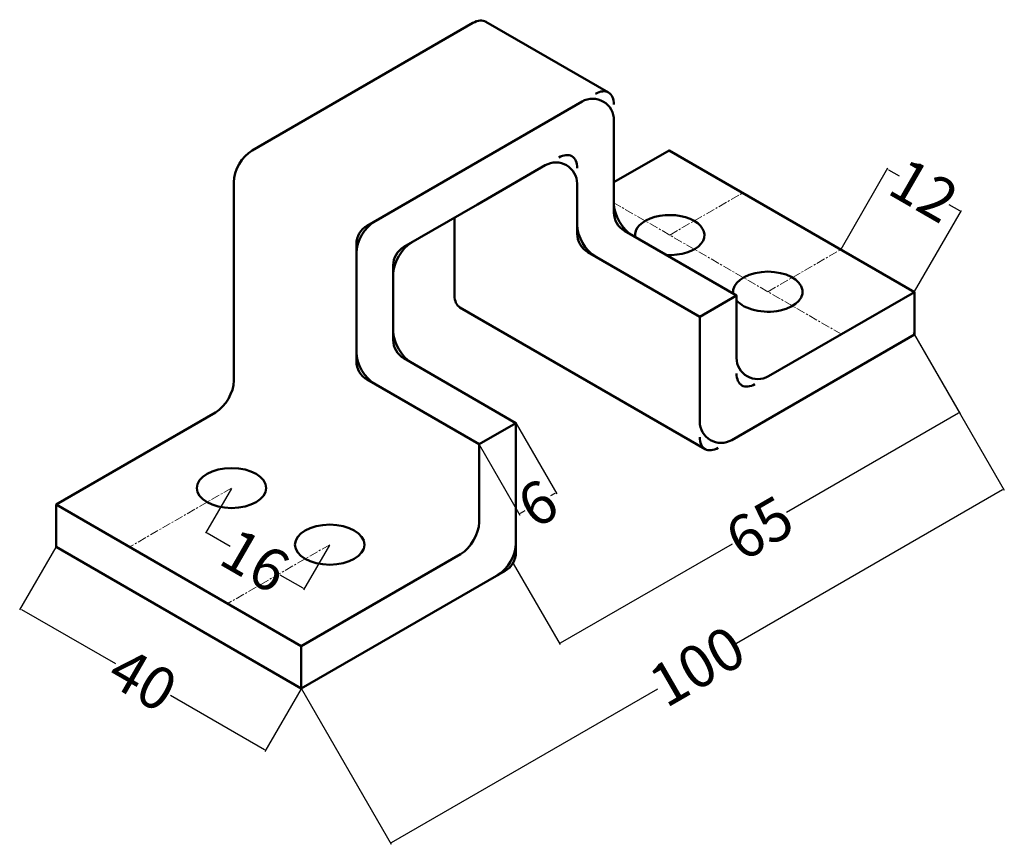
# Model space of a CAD drawing. Units: millimetres. Extents: x -15 to 124, y 15 to 131.
import ezdxf

# ---------------------------------------------------------------- set-up
doc = ezdxf.new("R2010")
doc.units = ezdxf.units.MM
doc.header["$MEASUREMENT"] = 0
doc.linetypes.add('CENTER', pattern=[2, 1.25, -0.25, 0.25, -0.25])
for name, color, linetype, lineweight in [('M-CNTR', 1, 'CENTER', 18), ('M-DIMS', 2, 'Continuous', 25), ('M-OUTL', 7, 'Continuous', 50)]:
    doc.layers.add(name, color=color, linetype=linetype, lineweight=lineweight)
doc.styles.get("Standard").update_dxf_attribs({"font": 'arial.ttf'})
doc.dimstyles.get("Standard").update_dxf_attribs({"dimtxt": 6, "dimasz": 0.18, "dimexe": 0.18, "dimexo": 0.0625, "dimgap": 0.09, "dimtad": 0, "dimtoh": 1, "dimdec": 0, "dimzin": 0, "dimdsep": 46, "dimtxsty": 'Standard', "dimcen": 0.09, "dimadec": 0, "dimazin": 0, "dimtfac": 1, "dimtdec": 0, "dimtofl": 0, "dimtmove": 0, "dimatfit": 3, "dimfxl": 1, "dimtolj": 1, "dimtzin": 0, "dimarcsym": 0})

# ---------------------------------------------------------------- blocks, each defined once
blk = doc.blocks.new('*D1')
at = {"layer": 'Defpoints', "color": 0, "transparency": 16777216}
for p in [(111.54, 86.71), (124.15, 64.87), (24.94, 36.71)]:
    blk.add_point(p, dxfattribs=at)
at = {"layer": 'M-DIMS', "color": 0, "lineweight": -2, "transparency": 16777216}
for p, q in [((111.57, 86.66), (124.24, 64.71)), ((123.99, 64.78), (86.41, 43.08)), ((24.97, 36.66), (37.64, 14.71)), ((37.7, 14.96), (75.28, 36.66))]:
    blk.add_line(p, q, dxfattribs=at)
at = {"layer": 'M-DIMS', "color": 0, "transparency": 16777216}
for points in [[(123.98, 64.81), (124.01, 64.75), (124.15, 64.87)], [(37.69, 14.99), (37.72, 14.93), (37.55, 14.87)]]:
    blk.add_solid(points, dxfattribs=at)
at = {"layer": 'M-DIMS', "color": 0, "transparency": 16777216, "insert": (80.85, 39.87), "char_height": 6, "attachment_point": 5, "rotation": 30}
blk.add_mtext('\\A1;100', dxfattribs=at)
blk = doc.blocks.new('*D2')
at = {"layer": 'Defpoints', "color": 0, "transparency": 16777216}
for p in [(111.34, 87.06), (117.91, 75.69), (54.85, 54.44)]:
    blk.add_point(p, dxfattribs=at)
at = {"layer": 'M-DIMS', "color": 0, "lineweight": -2, "transparency": 16777216}
for p, q in [((111.37, 87.01), (118, 75.53)), ((117.75, 75.6), (93.49, 61.59)), ((61.57, 43.16), (85.83, 57.16)), ((54.88, 54.39), (61.5, 42.91))]:
    blk.add_line(p, q, dxfattribs=at)
at = {"layer": 'M-DIMS', "color": 0, "transparency": 16777216}
for points in [[(117.73, 75.62), (117.76, 75.57), (117.91, 75.69)], [(61.55, 43.19), (61.58, 43.13), (61.41, 43.07)]]:
    blk.add_solid(points, dxfattribs=at)
at = {"layer": 'M-DIMS', "color": 0, "transparency": 16777216, "insert": (89.66, 59.38), "char_height": 6, "attachment_point": 5, "rotation": 30}
blk.add_mtext('\\A1;65', dxfattribs=at)
blk = doc.blocks.new('*D3')
at = {"layer": 'Defpoints', "color": 0, "transparency": 16777216}
for p in [(118.1, 104.07), (101.15, 98.71), (111.54, 92.71)]:
    blk.add_point(p, dxfattribs=at)
at = {"layer": 'M-DIMS', "color": 0, "lineweight": -2, "transparency": 16777216}
for p, q in [((101.18, 98.77), (107.79, 110.23)), ((107.86, 109.98), (109.37, 109.11)), ((117.94, 104.16), (116.43, 105.03)), ((111.57, 92.77), (118.19, 104.23))]:
    blk.add_line(p, q, dxfattribs=at)
at = {"layer": 'M-DIMS', "color": 0, "transparency": 16777216}
for points in [[(107.88, 110.01), (107.85, 109.95), (107.7, 110.07)], [(117.96, 104.19), (117.93, 104.13), (118.1, 104.07)]]:
    blk.add_solid(points, dxfattribs=at)
at = {"layer": 'M-DIMS', "color": 0, "transparency": 16777216, "insert": (112.9, 107.07), "char_height": 6, "attachment_point": 5, "rotation": 330}
blk.add_mtext('\\A1;12', dxfattribs=at)
blk = doc.blocks.new('*D4')
at = {"layer": 'Defpoints', "color": 0, "transparency": 16777216}
for p in [(15.09, 65.03), (28.95, 57.03), (25.35, 50.79)]:
    blk.add_point(p, dxfattribs=at)
at = {"layer": 'M-DIMS', "color": 0, "lineweight": -2, "transparency": 16777216}
for p, q in [((15.06, 64.97), (11.4, 58.64)), ((11.65, 58.7), (14.87, 56.84)), ((28.92, 56.97), (25.26, 50.64)), ((25.19, 50.88), (21.97, 52.74))]:
    blk.add_line(p, q, dxfattribs=at)
at = {"layer": 'M-DIMS', "color": 0, "transparency": 16777216}
for points in [[(11.66, 58.73), (11.63, 58.67), (11.49, 58.79)], [(25.21, 50.91), (25.18, 50.85), (25.35, 50.79)]]:
    blk.add_solid(points, dxfattribs=at)
at = {"layer": 'M-DIMS', "color": 0, "transparency": 16777216, "insert": (18.42, 54.79), "char_height": 6, "attachment_point": 5, "rotation": 330}
blk.add_mtext('\\A1;16', dxfattribs=at)
blk = doc.blocks.new('*D5')
at = {"layer": 'Defpoints', "color": 0, "transparency": 16777216}
for p in [(55.25, 74.21), (50.05, 71.21), (60.93, 64.37)]:
    blk.add_point(p, dxfattribs=at)
at = {"layer": 'M-DIMS', "color": 0, "lineweight": -2, "transparency": 16777216}
for p, q in [((55.28, 74.16), (61.02, 64.22)), ((50.08, 71.16), (55.82, 61.22)), ((60.77, 64.28), (60.12, 63.91)), ((55.89, 61.46), (56.54, 61.84))]:
    blk.add_line(p, q, dxfattribs=at)
at = {"layer": 'M-DIMS', "color": 0, "transparency": 16777216}
for points in [[(60.76, 64.31), (60.79, 64.26), (60.93, 64.37)], [(55.87, 61.49), (55.9, 61.44), (55.73, 61.37)]]:
    blk.add_solid(points, dxfattribs=at)
at = {"layer": 'M-DIMS', "color": 0, "transparency": 16777216, "insert": (58.33, 62.87), "char_height": 6, "attachment_point": 5, "rotation": 30}
blk.add_mtext('\\A1;6', dxfattribs=at)
blk = doc.blocks.new('*D6')
at = {"layer": 'Defpoints', "color": 0, "transparency": 16777216}
for p in [(-9.7, 56.71), (24.94, 36.71), (19.9, 27.98)]:
    blk.add_point(p, dxfattribs=at)
at = {"layer": 'M-DIMS', "color": 0, "lineweight": -2, "transparency": 16777216}
for p, q in [((-9.74, 56.66), (-14.84, 47.82)), ((-14.59, 47.89), (-1.32, 40.23)), ((24.91, 36.66), (19.81, 27.82)), ((19.74, 28.07), (6.47, 35.73))]:
    blk.add_line(p, q, dxfattribs=at)
at = {"layer": 'M-DIMS', "color": 0, "transparency": 16777216}
for points in [[(-14.57, 47.92), (-14.6, 47.86), (-14.75, 47.98)], [(19.75, 28.1), (19.72, 28.04), (19.9, 27.98)]]:
    blk.add_solid(points, dxfattribs=at)
at = {"layer": 'M-DIMS', "color": 0, "transparency": 16777216, "insert": (2.57, 37.98), "char_height": 6, "attachment_point": 5, "rotation": 330}
blk.add_mtext('\\A1;40', dxfattribs=at)

msp = doc.modelspace()

# ---------------------------------------------------------------- linework, layer by layer
at = {"layer": 'M-CNTR'}
for p, q in [((76.98, 100.76), (87.29, 106.71)), ((101.23, 86.76), (69.1, 105.31)), ((90.84, 92.76), (101.23, 98.76)), ((15.09, 65.03), (0.69, 56.71)), ((28.95, 57.03), (14.54, 48.71))]:
    msp.add_line(p, q, dxfattribs=at)
at = {"layer": 'M-OUTL'}
for p, q in [((68.34, 120.89), (51.02, 130.89)), ((18.01, 112.71), (49.19, 130.71)), ((15.41, 80.21), (15.41, 108.21)), ((46.59, 92.21), (46.59, 103.21)), ((81.99, 70.53), (47.35, 90.53)), ((-9.7, 62.71), (12.81, 75.71)), ((50.05, 60.21), (50.05, 71.21)), ((24.94, 42.71), (-9.7, 62.71)), ((24.94, 42.71), (47.45, 55.71))]:
    msp.add_line(p, q, dxfattribs=at)
for points in [[(69.1, 108.21), (76.9, 112.71), (111.54, 92.71), (90.92, 80.81, -0.57735), (86.42, 83.41), (86.42, 92.21), (81.23, 89.21), (65.41, 98.35, -0.267949), (63.91, 100.94), (63.91, 108.02, 0.57735), (59.41, 110.61), (49.82, 105.08), (39.43, 99.08, 0.267949), (37.93, 96.48), (37.93, 85.94, 0.267949), (39.43, 83.35), (55.25, 74.21), (50.05, 71.21), (34.23, 80.35, -0.267949), (32.73, 82.94), (32.73, 99.48, -0.267949), (34.23, 102.08), (64.6, 119.61), (64.6, 119.61, -0.583481), (69.1, 116.96), (69.1, 117.02), (69.1, 103.94, 0.267949), (70.6, 101.35), (86.42, 92.21)], [(111.54, 92.71), (111.54, 86.71), (85.73, 71.81), (85.73, 71.81, -0.57735), (81.23, 74.41), (81.23, 74.41), (81.23, 89.21)], [(24.94, 36.71), (53.75, 53.35, 0.267949), (55.25, 55.94), (55.25, 74.21)]]:
    msp.add_lwpolyline(points, format="xyb", dxfattribs=at)
msp.add_lwpolyline([(-9.7, 62.71), (-9.7, 56.71), (24.94, 36.71), (24.94, 42.71)], dxfattribs=at)
for centre, major_axis, start_param, end_param in [((49.19, 127.71), (1.84, 3.18), 0, 0.785398), ((66.51, 117.71), (1.84, 3.18), 0, 0.785398), ((66.51, 117.71), (1.84, 3.18), 5.497787, 6.283185), ((18.01, 109.71), (-1.84, -3.18), 3.926991, 5.497787), ((61.31, 108.71), (1.84, 3.18), 0, 0.785398), ((61.31, 108.71), (1.84, 3.18), 5.497787, 6.283185), ((71.7, 103.71), (-1.84, 3.18), 0.785398, 2.356194), ((76.98, 100.76), (-4.9, 0), 1.47024, 6.383742), ((35.33, 99.71), (-1.84, -3.18), 3.926991, 5.497787), ((66.51, 100.71), (-1.84, 3.18), 0.785398, 2.356194), ((40.53, 96.71), (1.84, 3.18), 0.785398, 2.356194), ((90.84, 92.76), (-4.9, 0), 0.448217, 6.383742), ((49.19, 93.71), (-1.84, -3.18), 5.497787, 6.283185), ((40.53, 85.71), (-1.84, 3.18), 0.785398, 2.356194), ((35.33, 82.71), (-1.84, 3.18), 0.785398, 2.356194), ((89.02, 82.71), (1.84, 3.18), 2.356194, 3.141593), ((12.81, 78.71), (1.84, 3.18), 3.926991, 5.497787), ((89.02, 82.71), (1.84, 3.18), 3.141593, 3.926991), ((83.83, 73.71), (-1.84, -3.18), 5.497787, 6.283185), ((83.83, 73.71), (-1.84, -3.18), 0, 0.785398), ((47.45, 58.71), (1.84, 3.18), 3.926991, 5.497787), ((52.65, 55.71), (1.84, 3.18), 3.926991, 5.497787)]:
    msp.add_ellipse(centre, major_axis=major_axis, ratio=0.57735, start_param=start_param, end_param=end_param, dxfattribs=at)
for centre in [(15.09, 65.03), (28.95, 57.03)]:
    msp.add_ellipse(centre, major_axis=(-4.9, 0), ratio=0.57735, dxfattribs=at)

# ---------------------------------------------------------------- dimensions: what is measured, and where the dimension line sits
at = {"layer": 'M-DIMS'}
for p1, p2, distance, picture, middle in [((101.15, 98.71), (111.54, 92.71), 13.12, '*D3', (112.9, 107.07)), ((24.94, 36.71), (111.54, 86.71), -25.22, '*D1', (80.85, 39.87)), ((54.85, 54.44), (111.34, 87.06), -13.13, '*D2', (89.66, 59.38)), ((50.05, 71.21), (55.25, 74.21), -11.36, '*D5', (58.33, 62.87)), ((15.09, 65.03), (28.95, 57.03), -7.2, '*D4', (18.42, 54.79)), ((-9.7, 56.71), (24.94, 36.71), -10.08, '*D6', (2.57, 37.98))]:
    dim = msp.add_aligned_dim(p1=p1, p2=p2, distance=distance, dimstyle='Standard', override={"dimclrd": 0, "dimclre": 0, "dimclrt": 0}, dxfattribs=at)
    dim.commit()
    dim.dimension.update_dxf_attribs({"geometry": picture, "text_midpoint": middle})

doc.saveas('drawing.dxf')
